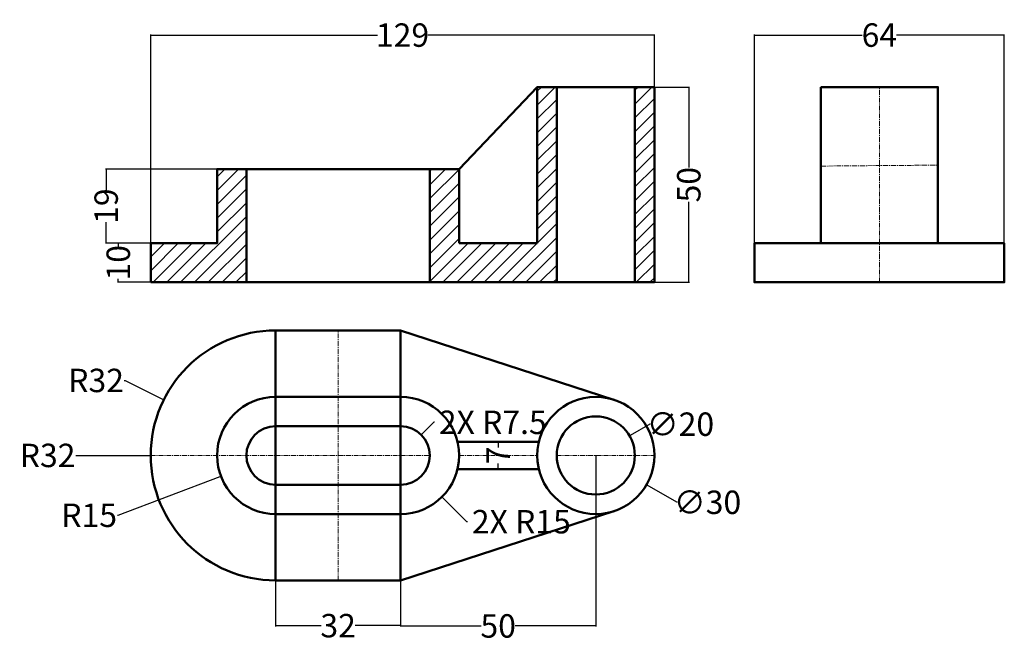
# Model space of a CAD drawing. Units: millimetres. Extents: x -9 to 243, y 7 to 166.
import ezdxf

# ---------------------------------------------------------------- set-up
doc = ezdxf.new("R2010")
doc.units = ezdxf.units.MM
doc.header["$MEASUREMENT"] = 0
doc.linetypes.add('CENTER', pattern=[2, 1.25, -0.25, 0.25, -0.25])
for name, color, linetype, lineweight in [('M-CNTR', 4, 'CENTER', 18), ('M-DIMS', 2, 'Continuous', 25), ('M-HATC', 8, 'Continuous', 18), ('M-OUTL', 7, 'Continuous', 50)]:
    doc.layers.add(name, color=color, linetype=linetype, lineweight=lineweight)
doc.styles.get("Standard").update_dxf_attribs({"font": 'arial.ttf'})
doc.dimstyles.get("Standard").update_dxf_attribs({"dimtxt": 6, "dimasz": 0.18, "dimexe": 0.18, "dimexo": 0.0625, "dimgap": 0.09, "dimtad": 0, "dimtoh": 1, "dimdec": 0, "dimzin": 0, "dimdsep": 46, "dimtxsty": 'Standard', "dimcen": 0.09, "dimadec": 0, "dimazin": 0, "dimtfac": 1, "dimtdec": 0, "dimtofl": 0, "dimtmove": 0, "dimatfit": 3, "dimfxl": 1, "dimtolj": 1, "dimtzin": 0, "dimarcsym": 0})

# ---------------------------------------------------------------- blocks, each defined once
blk = doc.blocks.new('*D1')
at = {"layer": 'Defpoints', "color": 0, "transparency": 16777216}
for p in [(153.23, 149.06), (153.23, 99.06), (162.05, 99.06)]:
    blk.add_point(p, dxfattribs=at)
at = {"layer": 'M-DIMS', "color": 0, "lineweight": -2, "transparency": 16777216}
for p, q in [((153.3, 149.06), (162.23, 149.06)), ((162.05, 148.88), (162.05, 128.44)), ((162.05, 99.24), (162.05, 119.69)), ((153.3, 99.06), (162.23, 99.06))]:
    blk.add_line(p, q, dxfattribs=at)
at = {"layer": 'M-DIMS', "color": 0, "transparency": 16777216}
for points in [[(162.02, 148.88), (162.08, 148.88), (162.05, 149.06)], [(162.02, 99.24), (162.08, 99.24), (162.05, 99.06)]]:
    blk.add_solid(points, dxfattribs=at)
at = {"layer": 'M-DIMS', "color": 0, "transparency": 16777216, "insert": (162.05, 124.06), "char_height": 6, "attachment_point": 5, "rotation": 90}
blk.add_mtext('\\A1;50', dxfattribs=at)
blk = doc.blocks.new('*D2')
at = {"layer": 'Defpoints', "color": 0, "transparency": 16777216}
for p in [(24.23, 109.06), (15.91, 99.06), (24.23, 99.06)]:
    blk.add_point(p, dxfattribs=at)
at = {"layer": 'M-DIMS', "color": 0, "lineweight": -2, "transparency": 16777216}
for p, q in [((24.17, 109.06), (15.73, 109.06)), ((15.91, 108.88), (15.91, 108.16)), ((24.17, 99.06), (15.73, 99.06)), ((15.91, 99.24), (15.91, 99.97))]:
    blk.add_line(p, q, dxfattribs=at)
at = {"layer": 'M-DIMS', "color": 0, "transparency": 16777216}
for points in [[(15.88, 108.88), (15.94, 108.88), (15.91, 109.06)], [(15.88, 99.24), (15.94, 99.24), (15.91, 99.06)]]:
    blk.add_solid(points, dxfattribs=at)
at = {"layer": 'M-DIMS', "color": 0, "transparency": 16777216, "insert": (15.91, 104.06), "char_height": 6, "attachment_point": 5, "rotation": 90}
blk.add_mtext('\\A1;10', dxfattribs=at)
blk = doc.blocks.new('*D3')
at = {"layer": 'Defpoints', "color": 0, "transparency": 16777216}
for p in [(41.23, 128.06), (12.81, 109.06), (41.23, 109.06)]:
    blk.add_point(p, dxfattribs=at)
at = {"layer": 'M-DIMS', "color": 0, "lineweight": -2, "transparency": 16777216}
for p, q in [((41.17, 128.06), (12.63, 128.06)), ((12.81, 127.88), (12.81, 122.68)), ((12.81, 109.24), (12.81, 114.45)), ((41.17, 109.06), (12.63, 109.06))]:
    blk.add_line(p, q, dxfattribs=at)
at = {"layer": 'M-DIMS', "color": 0, "transparency": 16777216}
for points in [[(12.78, 127.88), (12.84, 127.88), (12.81, 128.06)], [(12.78, 109.24), (12.84, 109.24), (12.81, 109.06)]]:
    blk.add_solid(points, dxfattribs=at)
at = {"layer": 'M-DIMS', "color": 0, "transparency": 16777216, "insert": (12.81, 118.56), "char_height": 6, "attachment_point": 5, "rotation": 90}
blk.add_mtext('\\A1;19', dxfattribs=at)
blk = doc.blocks.new('*D4')
at = {"layer": 'Defpoints', "color": 0, "transparency": 16777216}
for p in [(27.58, 68.98), (56.23, 54.73)]:
    blk.add_point(p, dxfattribs=at)
at = {"layer": 'M-DIMS', "color": 0, "lineweight": -2, "transparency": 16777216}
for p, q in [((17.46, 73.93), (17.64, 73.93)), ((17.64, 73.93), (27.42, 69.06)), ((56.14, 54.73), (56.32, 54.73)), ((56.23, 54.64), (56.23, 54.82))]:
    blk.add_line(p, q, dxfattribs=at)
at = {"layer": 'M-DIMS', "color": 0, "transparency": 16777216}
blk.add_solid([(27.44, 69.09), (27.41, 69.03), (27.58, 68.98)], dxfattribs=at)
at = {"layer": 'M-DIMS', "color": 0, "transparency": 16777216, "insert": (10.23, 73.93), "char_height": 6, "attachment_point": 5}
blk.add_mtext('\\A1;R32', dxfattribs=at)
blk = doc.blocks.new('*D5')
at = {"layer": 'Defpoints', "color": 0, "transparency": 16777216}
for p in [(56.23, 54.73), (42.21, 49.4)]:
    blk.add_point(p, dxfattribs=at)
at = {"layer": 'M-DIMS', "color": 0, "lineweight": -2, "transparency": 16777216}
for p, q in [((56.14, 54.73), (56.32, 54.73)), ((56.23, 54.64), (56.23, 54.82)), ((15.91, 39.41), (42.04, 49.34)), ((15.73, 39.41), (15.91, 39.41))]:
    blk.add_line(p, q, dxfattribs=at)
at = {"layer": 'M-DIMS', "color": 0, "transparency": 16777216}
blk.add_solid([(42.03, 49.37), (42.05, 49.31), (42.21, 49.4)], dxfattribs=at)
at = {"layer": 'M-DIMS', "color": 0, "transparency": 16777216, "insert": (8.45, 39.41), "char_height": 6, "attachment_point": 5}
blk.add_mtext('\\A1;R15', dxfattribs=at)
blk = doc.blocks.new('*D6')
at = {"layer": 'Defpoints', "color": 0, "transparency": 16777216}
for p in [(56.23, 22.73), (88.23, 22.73), (88.23, 11.14)]:
    blk.add_point(p, dxfattribs=at)
at = {"layer": 'M-DIMS', "color": 0, "lineweight": -2, "transparency": 16777216}
for p, q in [((56.23, 22.66), (56.23, 10.96)), ((88.23, 22.66), (88.23, 10.96)), ((56.41, 11.14), (67.88, 11.14)), ((88.05, 11.14), (76.59, 11.14))]:
    blk.add_line(p, q, dxfattribs=at)
at = {"layer": 'M-DIMS', "color": 0, "transparency": 16777216}
for points in [[(56.41, 11.17), (56.41, 11.11), (56.23, 11.14)], [(88.05, 11.17), (88.05, 11.11), (88.23, 11.14)]]:
    blk.add_solid(points, dxfattribs=at)
at = {"layer": 'M-DIMS', "color": 0, "transparency": 16777216, "insert": (72.23, 11.14), "char_height": 6, "attachment_point": 5}
blk.add_mtext('\\A1;32', dxfattribs=at)
blk = doc.blocks.new('*D7')
at = {"layer": 'Defpoints', "color": 0, "transparency": 16777216}
for p in [(113.23, 58.23), (113.23, 51.23), (113.23, 51.23)]:
    blk.add_point(p, dxfattribs=at)
at = {"layer": 'M-DIMS', "color": 0, "lineweight": -2, "transparency": 16777216}
for p, q in [((113.23, 58.05), (113.23, 56.76)), ((113.3, 58.23), (113.41, 58.23)), ((113.23, 51.41), (113.23, 52.69)), ((113.3, 51.23), (113.41, 51.23))]:
    blk.add_line(p, q, dxfattribs=at)
at = {"layer": 'M-DIMS', "color": 0, "transparency": 16777216}
for points in [[(113.2, 58.05), (113.26, 58.05), (113.23, 58.23)], [(113.2, 51.41), (113.26, 51.41), (113.23, 51.23)]]:
    blk.add_solid(points, dxfattribs=at)
at = {"layer": 'M-DIMS', "color": 0, "transparency": 16777216, "insert": (113.23, 54.73), "char_height": 6, "attachment_point": 5, "rotation": 90}
blk.add_mtext('\\A1;7', dxfattribs=at)
blk = doc.blocks.new('*D8')
at = {"layer": 'Defpoints', "color": 0, "transparency": 16777216}
for p in [(138.23, 54.73), (88.23, 22.73), (138.23, 11.07)]:
    blk.add_point(p, dxfattribs=at)
at = {"layer": 'M-DIMS', "color": 0, "lineweight": -2, "transparency": 16777216}
for p, q in [((138.23, 54.66), (138.23, 10.89)), ((88.23, 22.66), (88.23, 10.89)), ((88.41, 11.07), (108.86, 11.07)), ((138.05, 11.07), (117.61, 11.07))]:
    blk.add_line(p, q, dxfattribs=at)
at = {"layer": 'M-DIMS', "color": 0, "transparency": 16777216}
for points in [[(88.41, 11.1), (88.41, 11.04), (88.23, 11.07)], [(138.05, 11.1), (138.05, 11.04), (138.23, 11.07)]]:
    blk.add_solid(points, dxfattribs=at)
at = {"layer": 'M-DIMS', "color": 0, "transparency": 16777216, "insert": (113.23, 11.07), "char_height": 6, "attachment_point": 5}
blk.add_mtext('\\A1;50', dxfattribs=at)
blk = doc.blocks.new('*D9')
at = {"layer": 'Defpoints', "color": 0, "transparency": 16777216}
for p in [(153.23, 162.36), (153.23, 149.06), (24.23, 109.06)]:
    blk.add_point(p, dxfattribs=at)
at = {"layer": 'M-DIMS', "color": 0, "lineweight": -2, "transparency": 16777216}
for p, q in [((24.23, 109.13), (24.23, 162.54)), ((24.41, 162.36), (82.29, 162.36)), ((153.05, 162.36), (95.18, 162.36)), ((153.23, 149.13), (153.23, 162.54))]:
    blk.add_line(p, q, dxfattribs=at)
at = {"layer": 'M-DIMS', "color": 0, "transparency": 16777216}
for points in [[(24.41, 162.39), (24.41, 162.33), (24.23, 162.36)], [(153.05, 162.39), (153.05, 162.33), (153.23, 162.36)]]:
    blk.add_solid(points, dxfattribs=at)
at = {"layer": 'M-DIMS', "color": 0, "transparency": 16777216, "insert": (88.73, 162.36), "char_height": 6, "attachment_point": 5}
blk.add_mtext('\\A1;129', dxfattribs=at)
blk = doc.blocks.new('*D10')
at = {"layer": 'Defpoints', "color": 0, "transparency": 16777216}
for p in [(242.87, 162.36), (178.87, 109.06), (242.87, 109.06)]:
    blk.add_point(p, dxfattribs=at)
at = {"layer": 'M-DIMS', "color": 0, "lineweight": -2, "transparency": 16777216}
for p, q in [((178.87, 109.13), (178.87, 162.54)), ((179.05, 162.36), (206.48, 162.36)), ((242.69, 162.36), (215.26, 162.36)), ((242.87, 109.13), (242.87, 162.54))]:
    blk.add_line(p, q, dxfattribs=at)
at = {"layer": 'M-DIMS', "color": 0, "transparency": 16777216}
for points in [[(179.05, 162.39), (179.05, 162.33), (178.87, 162.36)], [(242.69, 162.39), (242.69, 162.33), (242.87, 162.36)]]:
    blk.add_solid(points, dxfattribs=at)
at = {"layer": 'M-DIMS', "color": 0, "transparency": 16777216, "insert": (210.87, 162.36), "char_height": 6, "attachment_point": 5}
blk.add_mtext('\\A1;64', dxfattribs=at)
blk = doc.blocks.new('*D11')
at = {"layer": 'Defpoints', "color": 0, "transparency": 16777216}
for p in [(24.23, 54.73), (56.23, 54.73)]:
    blk.add_point(p, dxfattribs=at)
at = {"layer": 'M-DIMS', "color": 0, "lineweight": -2, "transparency": 16777216}
for p, q in [((5.03, 54.73), (24.05, 54.73)), ((56.14, 54.73), (56.32, 54.73)), ((56.23, 54.64), (56.23, 54.82))]:
    blk.add_line(p, q, dxfattribs=at)
at = {"layer": 'M-DIMS', "color": 0, "transparency": 16777216}
blk.add_solid([(24.05, 54.76), (24.05, 54.7), (24.23, 54.73)], dxfattribs=at)
at = {"layer": 'M-DIMS', "color": 0, "transparency": 16777216, "insert": (-2.19, 54.73), "char_height": 6, "attachment_point": 5}
blk.add_mtext('\\A1;R32', dxfattribs=at)
blk = doc.blocks.new('*D12')
at = {"layer": 'Defpoints', "color": 0, "transparency": 16777216}
for p in [(88.23, 54.73), (98.84, 44.12)]:
    blk.add_point(p, dxfattribs=at)
at = {"layer": 'M-DIMS', "color": 0, "lineweight": -2, "transparency": 16777216}
for p, q in [((88.14, 54.73), (88.32, 54.73)), ((88.23, 54.64), (88.23, 54.82)), ((105.2, 37.76), (98.97, 43.99)), ((105.38, 37.76), (105.2, 37.76))]:
    blk.add_line(p, q, dxfattribs=at)
at = {"layer": 'M-DIMS', "color": 0, "transparency": 16777216}
blk.add_solid([(98.99, 44.01), (98.95, 43.97), (98.84, 44.12)], dxfattribs=at)
at = {"layer": 'M-DIMS', "color": 0, "transparency": 16777216, "insert": (119.16, 37.76), "char_height": 6, "attachment_point": 5}
blk.add_mtext('\\A1;2X R15', dxfattribs=at)
blk = doc.blocks.new('*D13')
at = {"layer": 'Defpoints', "color": 0, "transparency": 16777216}
for p in [(93.54, 60.03), (88.23, 54.73)]:
    blk.add_point(p, dxfattribs=at)
at = {"layer": 'M-DIMS', "color": 0, "lineweight": -2, "transparency": 16777216}
for p, q in [((96.72, 63.21), (93.66, 60.16)), ((96.9, 63.21), (96.72, 63.21)), ((88.14, 54.73), (88.32, 54.73)), ((88.23, 54.64), (88.23, 54.82))]:
    blk.add_line(p, q, dxfattribs=at)
at = {"layer": 'M-DIMS', "color": 0, "transparency": 16777216}
blk.add_solid([(93.64, 60.18), (93.69, 60.14), (93.54, 60.03)], dxfattribs=at)
at = {"layer": 'M-DIMS', "color": 0, "transparency": 16777216, "insert": (111.84, 63.21), "char_height": 6, "attachment_point": 5}
blk.add_mtext('\\A1;2X R7.5', dxfattribs=at)
blk = doc.blocks.new('*D14')
at = {"layer": 'Defpoints', "color": 0, "transparency": 16777216}
for p in [(146.89, 59.73), (129.57, 49.73)]:
    blk.add_point(p, dxfattribs=at)
at = {"layer": 'M-DIMS', "color": 0, "lineweight": -2, "transparency": 16777216}
for p, q in [((152.09, 62.73), (147.05, 59.82)), ((152.27, 62.73), (152.09, 62.73)), ((138.14, 54.73), (138.32, 54.73)), ((138.23, 54.64), (138.23, 54.82))]:
    blk.add_line(p, q, dxfattribs=at)
at = {"layer": 'M-DIMS', "color": 0, "transparency": 16777216}
blk.add_solid([(147.04, 59.84), (147.07, 59.79), (146.89, 59.73)], dxfattribs=at)
at = {"layer": 'M-DIMS', "color": 0, "transparency": 16777216, "insert": (159.91, 62.73), "char_height": 6, "attachment_point": 5}
blk.add_mtext('\\A1;∅20', dxfattribs=at)
blk = doc.blocks.new('*D15')
at = {"layer": 'Defpoints', "color": 0, "transparency": 16777216}
for p in [(125.24, 62.23), (151.22, 47.23)]:
    blk.add_point(p, dxfattribs=at)
at = {"layer": 'M-DIMS', "color": 0, "lineweight": -2, "transparency": 16777216}
for p, q in [((138.14, 54.73), (138.32, 54.73)), ((138.23, 54.64), (138.23, 54.82)), ((159.02, 42.73), (151.38, 47.14)), ((159.2, 42.73), (159.02, 42.73))]:
    blk.add_line(p, q, dxfattribs=at)
at = {"layer": 'M-DIMS', "color": 0, "transparency": 16777216}
blk.add_solid([(151.4, 47.16), (151.37, 47.11), (151.22, 47.23)], dxfattribs=at)
at = {"layer": 'M-DIMS', "color": 0, "transparency": 16777216, "insert": (166.84, 42.73), "char_height": 6, "attachment_point": 5}
blk.add_mtext('\\A1;∅30', dxfattribs=at)

msp = doc.modelspace()

# ---------------------------------------------------------------- hatches: boundary and pattern name
at = {"layer": 'M-HATC'}
h = msp.add_hatch(dxfattribs=at)
h.set_pattern_fill('ANSI31', color=256, scale=20)
h.paths.add_polyline_path([(48.73, 128.06), (41.23, 128.06), (41.23, 109.06), (24.23, 109.06), (24.23, 99.06), (48.73, 99.06)])
h.paths.add_polyline_path([(103.23, 128.06), (95.73, 128.06), (95.73, 99.06), (128.23, 99.06), (128.23, 149.06), (123.23, 149.06), (123.23, 109.06), (103.23, 109.06)])
h.paths.add_polyline_path([(153.23, 149.06), (148.23, 149.06), (148.23, 99.06), (153.23, 99.06)])

# ---------------------------------------------------------------- linework, layer by layer
at = {"layer": 'M-CNTR'}
for p, q in [((210.87, 99.06), (210.87, 149.06)), ((195.87, 128.82), (225.87, 129.06)), ((72.23, 22.73), (72.23, 86.73)), ((24.23, 54.73), (95.73, 54.73)), ((103.23, 54.73), (123.23, 54.73)), ((128.23, 54.73), (153.23, 54.73))]:
    msp.add_line(p, q, dxfattribs=at)
at = {"layer": 'M-OUTL'}
for p, q in [((123.23, 109.06), (123.23, 149.06)), ((128.23, 99.06), (128.23, 149.06)), ((148.23, 99.06), (148.23, 149.06)), ((48.73, 99.06), (48.73, 128.06)), ((95.73, 99.06), (95.73, 128.06)), ((103.23, 109.06), (103.23, 128.06)), ((123.23, 109.06), (103.23, 109.06)), ((102.82, 58.23), (123.65, 58.23)), ((102.82, 51.23), (123.65, 51.23))]:
    msp.add_line(p, q, dxfattribs=at)
for points in [[(24.23, 99.06), (24.23, 109.06), (41.23, 109.06), (41.23, 128.06), (48.73, 128.06), (95.73, 128.06), (103.23, 128.06), (123.23, 149.06), (153.23, 149.06), (153.23, 99.06)], [(195.87, 149.06), (195.87, 109.06), (225.87, 109.06), (225.87, 149.06), (210.87, 149.06)]]:
    msp.add_lwpolyline(points, close=True, dxfattribs=at)
for points in [[(225.87, 109.06), (242.87, 109.06), (242.87, 99.06), (178.87, 99.06), (178.87, 109.06), (195.87, 109.06)], [(88.23, 86.73), (56.23, 86.73), (56.23, 22.73), (88.23, 22.73)], [(142.87, 68.99), (88.23, 86.73), (88.23, 22.73), (142.87, 40.46)]]:
    msp.add_lwpolyline(points, dxfattribs=at)
for points in [[(56.23, 39.73), (88.23, 39.73, 1), (88.23, 69.73), (56.23, 69.73, 1)], [(56.23, 47.23), (88.23, 47.23, 1), (88.23, 62.23), (56.23, 62.23, 1)]]:
    msp.add_lwpolyline(points, format="xyb", close=True, dxfattribs=at)
for radius in [15, 10]:
    msp.add_circle((138.23, 54.73), radius, dxfattribs=at)
msp.add_arc((56.23, 54.73), 32, 90, 270, dxfattribs=at)

# ---------------------------------------------------------------- dimensions: what is measured, and where the dimension line sits
at = {"layer": 'M-DIMS'}
for base, p1, p2, override, picture, middle in [((153.23, 162.36), (24.23, 109.06), (153.23, 149.06), {"dimdec": 0, "dimlfac": 1, "dimrnd": 0, "dimzin": 0, "dimdsep": 46, "dimlunit": 2}, '*D9', (88.73, 162.36)), ((242.87, 162.36), (178.87, 109.06), (242.87, 109.06), {"dimdec": 0, "dimlfac": 1, "dimrnd": 0, "dimzin": 0, "dimdsep": 46, "dimlunit": 2}, '*D10', (210.87, 162.36)), ((138.23, 11.07), (88.23, 22.73), (138.23, 54.73), {"dimclrd": 0, "dimclre": 0, "dimclrt": 0}, '*D8', (113.23, 11.07)), ((88.23, 11.14), (56.23, 22.73), (88.23, 22.73), {"dimclrd": 0, "dimclre": 0, "dimclrt": 0}, '*D6', (72.23, 11.14))]:
    dim = msp.add_linear_dim(base=base, p1=p1, p2=p2, dimstyle='Standard', override=override, dxfattribs=at)
    dim.commit()
    dim.dimension.update_dxf_attribs({"geometry": picture, "text_midpoint": middle})
for base, p1, p2, picture, middle in [((162.05, 99.06), (153.23, 149.06), (153.23, 99.06), '*D1', (162.05, 124.06)), ((12.81, 109.06), (41.23, 128.06), (41.23, 109.06), '*D3', (12.81, 118.56)), ((15.91, 99.06), (24.23, 109.06), (24.23, 99.06), '*D2', (15.91, 104.06)), ((113.23, 51.23), (113.23, 58.23), (113.23, 51.23), '*D7', (113.23, 54.73))]:
    dim = msp.add_linear_dim(base=base, p1=p1, p2=p2, angle=90, dimstyle='Standard', override={"dimclrd": 0, "dimclre": 0, "dimclrt": 0}, dxfattribs=at)
    dim.commit()
    dim.dimension.update_dxf_attribs({"geometry": picture, "text_midpoint": middle})
for mpoint, override, picture, middle in [((27.58, 68.98), {"dimclrd": 0, "dimclre": 0, "dimclrt": 0}, '*D4', (10.23, 73.93)), ((24.23, 54.73), {"dimdec": 0, "dimlfac": 1, "dimrnd": 0, "dimzin": 0, "dimdsep": 46, "dimlunit": 2}, '*D11', (5.03, 54.73)), ((42.21, 49.4), {"dimclrd": 0, "dimclre": 0, "dimclrt": 0}, '*D5', (8.45, 39.41))]:
    dim = msp.add_radius_dim(center=(56.23, 54.73), mpoint=mpoint, dimstyle='Standard', override=override, dxfattribs=at)
    dim.commit()
    dim.dimension.update_dxf_attribs({"geometry": picture, "text_midpoint": middle, "dimtype": 164})
for mpoint, override, picture, middle in [((93.54, 60.03), {"dimdec": 1, "dimlfac": 1, "dimrnd": 0, "dimzin": 0, "dimdsep": 46, "dimlunit": 2}, '*D13', (111.84, 63.21)), ((98.84, 44.12), {"dimdec": 0, "dimlfac": 1, "dimrnd": 0, "dimzin": 0, "dimdsep": 46, "dimlunit": 2}, '*D12', (119.16, 37.76))]:
    dim = msp.add_radius_dim(center=(88.23, 54.73), mpoint=mpoint, text='2X <>', dimstyle='Standard', override=override, dxfattribs=at)
    dim.commit()
    dim.dimension.update_dxf_attribs({"geometry": picture, "text_midpoint": middle, "dimtype": 164})
for p1, p2, picture, middle in [((129.57, 49.73), (146.89, 59.73), '*D14', (159.91, 62.73)), ((125.24, 62.23), (151.22, 47.23), '*D15', (166.84, 42.73))]:
    dim = msp.add_diameter_dim_2p(p1=p1, p2=p2, dimstyle='Standard', override={"dimdec": 0, "dimlfac": 1, "dimrnd": 0, "dimzin": 0, "dimdsep": 46, "dimlunit": 2}, dxfattribs=at)
    dim.commit()
    dim.dimension.update_dxf_attribs({"geometry": picture, "text_midpoint": middle, "dimtype": 163})

doc.saveas('drawing.dxf')
